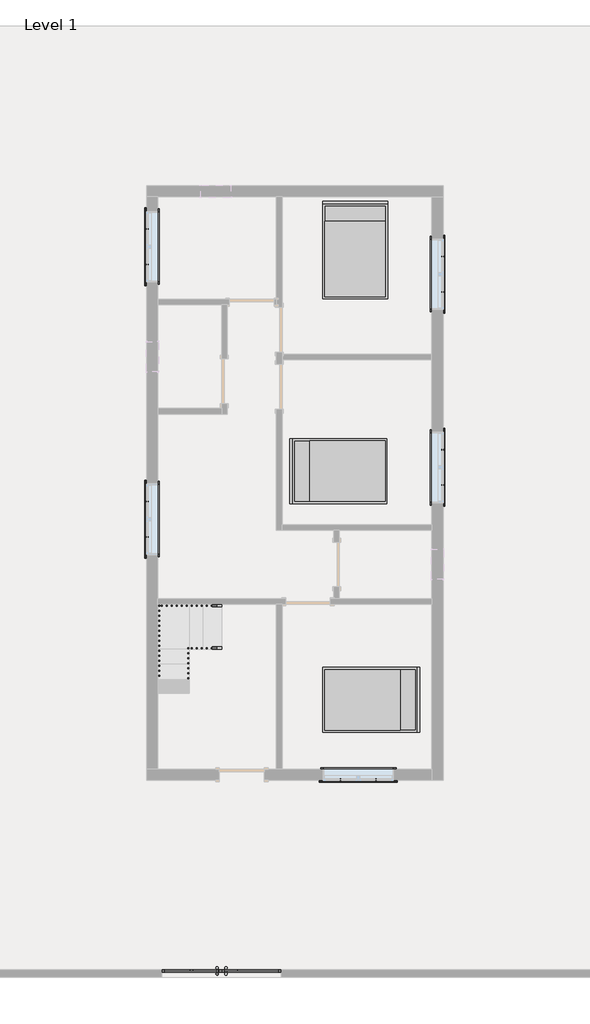
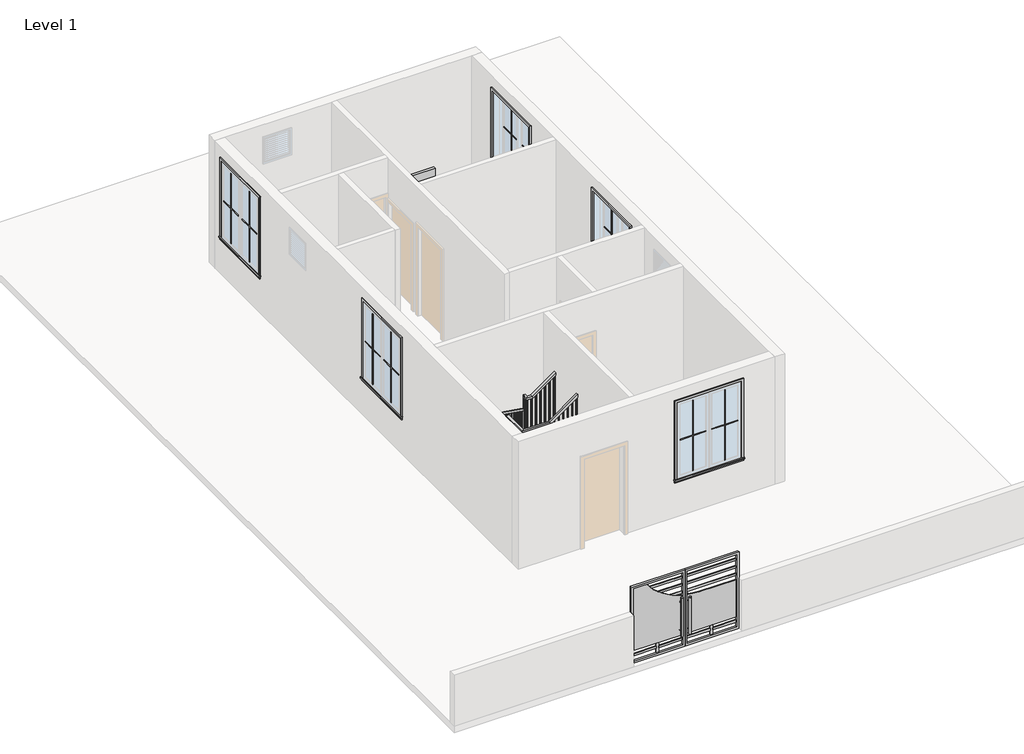
# One storey, part 2 of 2: 21 proxies, 3 furniture elements, 2 railings.
"""IFC4 building model written with IfcOpenShell, lengths in millimetres."""

from ifc_helpers import new_model, si_unit, frame, origin, place, context, project, spatial, polyline, outline, extrude, faceted_brep, transform, mapped, element, save
from components import generic_models_113f6068, muntin_pattern_2x2_muntin_pattern_2x2_bff912c5, muntin_pattern_2x2_muntin_pattern_2x2_c2194282, trim_window_exterior_flat_with_sill_e04b3088, trim_window_interior_flat_picture_frame_2a7685fe, bed_17739_bed_17739_15c61121

model = new_model("IFC4")

# Units and contexts
model_context = context("Model", 3, world=origin())
ifc_project = project(units=[si_unit("LENGTHUNIT", "METRE", prefix="MILLI")], contexts=[model_context])

# Site, building, storey
site = spatial("IfcSite", under=ifc_project)
building = spatial("IfcBuilding", under=site)
storey = spatial("IfcBuildingStorey", under=building, Name="Level 1", Elevation=0.0)

# Proxies
placement = place(None, origin())
generic_models_shape = generic_models_113f6068(model_context)
element("IfcBuildingElementProxy", 1, Name="Generic Models", at=placement, inside=storey, context=model_context, shape_type="MappedRepresentation", body=[
    mapped(generic_models_shape, transform((-2747.4889285, -9775.3328853, 0.0), x_axis=(1.0, 0.0, 0.0), y_axis=(0.0, 1.0, 0.0), z_axis=(0.0, 0.0, 1.0))),
])
muntin_pattern_2x2_muntin_pattern_2x2_shape = muntin_pattern_2x2_muntin_pattern_2x2_bff912c5(model_context)
element("IfcBuildingElementProxy", 2, Name="Muntin Pattern_2x2 : Muntin Pattern_2x2", ObjectType="Muntin Pattern_2x2 : Muntin Pattern_2x2", at=placement, inside=storey, context=model_context, shape_type="MappedRepresentation", body=[
    mapped(muntin_pattern_2x2_muntin_pattern_2x2_shape, transform((-4261.9639285, 4584.2694249, 984.25), x_axis=(0.0, 1.0, 0.0), y_axis=(-1.0, 0.0, 0.0), z_axis=(0.0, 0.0, 1.0))),
])
element("IfcBuildingElementProxy", 3, Name="Muntin Pattern_2x2 : Muntin Pattern_2x2", ObjectType="Muntin Pattern_2x2 : Muntin Pattern_2x2", at=placement, inside=storey, context=model_context, shape_type="MappedRepresentation", body=[
    mapped(muntin_pattern_2x2_muntin_pattern_2x2_shape, transform((1751.4860715, 4746.1944249, 984.25), x_axis=(0.0, -1.0, 0.0), y_axis=(1.0, 0.0, 0.0), z_axis=(0.0, 0.0, 1.0))),
])
element("IfcBuildingElementProxy", 4, Name="Muntin Pattern_2x2 : Muntin Pattern_2x2", ObjectType="Muntin Pattern_2x2 : Muntin Pattern_2x2", at=placement, inside=storey, context=model_context, shape_type="MappedRepresentation", body=[
    mapped(muntin_pattern_2x2_muntin_pattern_2x2_shape, transform((-4261.9639285, -962.4555751, 984.25), x_axis=(0.0, 1.0, 0.0), y_axis=(-1.0, 0.0, 0.0), z_axis=(0.0, 0.0, 1.0))),
])
element("IfcBuildingElementProxy", 5, Name="Muntin Pattern_2x2 : Muntin Pattern_2x2", ObjectType="Muntin Pattern_2x2 : Muntin Pattern_2x2", at=placement, inside=storey, context=model_context, shape_type="MappedRepresentation", body=[
    mapped(muntin_pattern_2x2_muntin_pattern_2x2_shape, transform((1751.4860715, 812.3694249, 984.25), x_axis=(0.0, -1.0, 0.0), y_axis=(1.0, 0.0, 0.0), z_axis=(0.0, 0.0, 1.0))),
])
element("IfcBuildingElementProxy", 6, Name="Muntin Pattern_2x2 : Muntin Pattern_2x2", ObjectType="Muntin Pattern_2x2 : Muntin Pattern_2x2", at=placement, inside=storey, context=model_context, shape_type="MappedRepresentation", body=[
    mapped(muntin_pattern_2x2_muntin_pattern_2x2_shape, transform((397.3485715, -5907.5180751, 984.25), x_axis=(-1.0, 0.0, 0.0), y_axis=(0.0, -1.0, 0.0), z_axis=(0.0, 0.0, 1.0))),
])
muntin_pattern_2x2_muntin_pattern_2x2_2_shape = muntin_pattern_2x2_muntin_pattern_2x2_c2194282(model_context)
element("IfcBuildingElementProxy", 7, Name="Muntin Pattern_2x2 : Muntin Pattern_2x2", ObjectType="Muntin Pattern_2x2 : Muntin Pattern_2x2", at=placement, inside=storey, context=model_context, shape_type="MappedRepresentation", body=[
    mapped(muntin_pattern_2x2_muntin_pattern_2x2_2_shape, transform((-4261.9639285, 5304.9944249, 984.25), x_axis=(0.0, -1.0, 0.0), y_axis=(1.0, 0.0, 0.0), z_axis=(0.0, 0.0, 1.0))),
])
element("IfcBuildingElementProxy", 8, Name="Muntin Pattern_2x2 : Muntin Pattern_2x2", ObjectType="Muntin Pattern_2x2 : Muntin Pattern_2x2", at=placement, inside=storey, context=model_context, shape_type="MappedRepresentation", body=[
    mapped(muntin_pattern_2x2_muntin_pattern_2x2_2_shape, transform((1751.4860715, 4025.4694249, 984.25), x_axis=(0.0, 1.0, 0.0), y_axis=(-1.0, 0.0, 0.0), z_axis=(0.0, 0.0, 1.0))),
])
element("IfcBuildingElementProxy", 9, Name="Muntin Pattern_2x2 : Muntin Pattern_2x2", ObjectType="Muntin Pattern_2x2 : Muntin Pattern_2x2", at=placement, inside=storey, context=model_context, shape_type="MappedRepresentation", body=[
    mapped(muntin_pattern_2x2_muntin_pattern_2x2_2_shape, transform((-4261.9639285, -241.7305751, 984.25), x_axis=(0.0, -1.0, 0.0), y_axis=(1.0, 0.0, 0.0), z_axis=(0.0, 0.0, 1.0))),
])
element("IfcBuildingElementProxy", 10, Name="Muntin Pattern_2x2 : Muntin Pattern_2x2", ObjectType="Muntin Pattern_2x2 : Muntin Pattern_2x2", at=placement, inside=storey, context=model_context, shape_type="MappedRepresentation", body=[
    mapped(muntin_pattern_2x2_muntin_pattern_2x2_2_shape, transform((1751.4860715, 91.6444249, 984.25), x_axis=(0.0, 1.0, 0.0), y_axis=(-1.0, 0.0, 0.0), z_axis=(0.0, 0.0, 1.0))),
])
element("IfcBuildingElementProxy", 11, Name="Muntin Pattern_2x2 : Muntin Pattern_2x2", ObjectType="Muntin Pattern_2x2 : Muntin Pattern_2x2", at=placement, inside=storey, context=model_context, shape_type="MappedRepresentation", body=[
    mapped(muntin_pattern_2x2_muntin_pattern_2x2_2_shape, transform((-323.3764285, -5907.5180751, 984.25), x_axis=(1.0, 0.0, 0.0), y_axis=(0.0, 1.0, 0.0), z_axis=(0.0, 0.0, 1.0))),
])
trim_window_exterior_flat_with_sill_shape = trim_window_exterior_flat_with_sill_e04b3088(model_context)
element("IfcBuildingElementProxy", 12, Name="Trim-Window-Exterior-Flat : with Sill", ObjectType="Trim-Window-Exterior-Flat : with Sill", at=placement, inside=storey, context=model_context, shape_type="MappedRepresentation", body=[
    mapped(trim_window_exterior_flat_with_sill_shape, transform((-4271.4889285, 4944.6319249, 2743.2), x_axis=(0.0, -1.0, 0.0), y_axis=(0.0, 0.0, 1.0), z_axis=(-1.0, 0.0, 0.0))),
])
element("IfcBuildingElementProxy", 13, Name="Trim-Window-Exterior-Flat : with Sill", ObjectType="Trim-Window-Exterior-Flat : with Sill", at=placement, inside=storey, context=model_context, shape_type="MappedRepresentation", body=[
    mapped(trim_window_exterior_flat_with_sill_shape, transform((1761.0110715, 4385.8319249, 2743.2), x_axis=(0.0, 1.0, 0.0), y_axis=(0.0, 0.0, 1.0), z_axis=(1.0, 0.0, 0.0))),
])
element("IfcBuildingElementProxy", 14, Name="Trim-Window-Exterior-Flat : with Sill", ObjectType="Trim-Window-Exterior-Flat : with Sill", at=placement, inside=storey, context=model_context, shape_type="MappedRepresentation", body=[
    mapped(trim_window_exterior_flat_with_sill_shape, transform((-4271.4889285, -602.0930751, 2743.2), x_axis=(0.0, -1.0, 0.0), y_axis=(0.0, 0.0, 1.0), z_axis=(-1.0, 0.0, 0.0))),
])
element("IfcBuildingElementProxy", 15, Name="Trim-Window-Exterior-Flat : with Sill", ObjectType="Trim-Window-Exterior-Flat : with Sill", at=placement, inside=storey, context=model_context, shape_type="MappedRepresentation", body=[
    mapped(trim_window_exterior_flat_with_sill_shape, transform((1761.0110715, 452.0069249, 2743.2), x_axis=(0.0, 1.0, 0.0), y_axis=(0.0, 0.0, 1.0), z_axis=(1.0, 0.0, 0.0))),
])
element("IfcBuildingElementProxy", 16, Name="Trim-Window-Exterior-Flat : with Sill", ObjectType="Trim-Window-Exterior-Flat : with Sill", at=placement, inside=storey, context=model_context, shape_type="MappedRepresentation", body=[
    mapped(trim_window_exterior_flat_with_sill_shape, transform((36.9860715, -5917.0430751, 2743.2), x_axis=(1.0, 0.0, 0.0), y_axis=(0.0, 0.0, 1.0), z_axis=(0.0, -1.0, 0.0))),
])
trim_window_interior_flat_picture_frame_shape = trim_window_interior_flat_picture_frame_2a7685fe(model_context)
element("IfcBuildingElementProxy", 17, Name="Trim-Window-Interior-Flat : Picture Frame", ObjectType="Trim-Window-Interior-Flat : Picture Frame", at=placement, inside=storey, context=model_context, shape_type="MappedRepresentation", body=[
    mapped(trim_window_interior_flat_picture_frame_shape, transform((-4042.8889285, 4944.6319249, 2743.2), x_axis=(0.0, 1.0, 0.0), y_axis=(0.0, 0.0, 1.0), z_axis=(1.0, 0.0, 0.0))),
])
element("IfcBuildingElementProxy", 18, Name="Trim-Window-Interior-Flat : Picture Frame", ObjectType="Trim-Window-Interior-Flat : Picture Frame", at=placement, inside=storey, context=model_context, shape_type="MappedRepresentation", body=[
    mapped(trim_window_interior_flat_picture_frame_shape, transform((1532.4110715, 4385.8319249, 2743.2), x_axis=(0.0, -1.0, 0.0), y_axis=(0.0, 0.0, 1.0), z_axis=(-1.0, 0.0, 0.0))),
])
element("IfcBuildingElementProxy", 19, Name="Trim-Window-Interior-Flat : Picture Frame", ObjectType="Trim-Window-Interior-Flat : Picture Frame", at=placement, inside=storey, context=model_context, shape_type="MappedRepresentation", body=[
    mapped(trim_window_interior_flat_picture_frame_shape, transform((-4042.8889285, -602.0930751, 2743.2), x_axis=(0.0, 1.0, 0.0), y_axis=(0.0, 0.0, 1.0), z_axis=(1.0, 0.0, 0.0))),
])
element("IfcBuildingElementProxy", 20, Name="Trim-Window-Interior-Flat : Picture Frame", ObjectType="Trim-Window-Interior-Flat : Picture Frame", at=placement, inside=storey, context=model_context, shape_type="MappedRepresentation", body=[
    mapped(trim_window_interior_flat_picture_frame_shape, transform((1532.4110715, 452.0069249, 2743.2), x_axis=(0.0, -1.0, 0.0), y_axis=(0.0, 0.0, 1.0), z_axis=(-1.0, 0.0, 0.0))),
])
element("IfcBuildingElementProxy", 21, Name="Trim-Window-Interior-Flat : Picture Frame", ObjectType="Trim-Window-Interior-Flat : Picture Frame", at=placement, inside=storey, context=model_context, shape_type="MappedRepresentation", body=[
    mapped(trim_window_interior_flat_picture_frame_shape, transform((36.9860715, -5688.4430751, 2743.2), x_axis=(-1.0, 0.0, 0.0), y_axis=(0.0, 0.0, 1.0), z_axis=(0.0, 1.0, 0.0))),
])

# Furniture
bed_17739_bed_17739_shape = bed_17739_bed_17739_15c61121(model_context)
element("IfcFurniture", 22, ObjectType="Bed_17739 : Bed_17739", at=placement, inside=storey, context=model_context, shape_type="MappedRepresentation", body=[
    mapped(bed_17739_bed_17739_shape, transform((-29.6889285, 4852.5569249, 0.0), x_axis=(1.0, 0.0, 0.0), y_axis=(0.0, 1.0, 0.0), z_axis=(0.0, 0.0, 1.0))),
])
element("IfcFurniture", 23, ObjectType="Bed_17739 : Bed_17739", at=placement, inside=storey, context=model_context, shape_type="MappedRepresentation", body=[
    mapped(bed_17739_bed_17739_shape, transform((-347.1889285, 375.8069249, 0.0), x_axis=(0.0, 1.0, 0.0), y_axis=(-1.0, 0.0, 0.0), z_axis=(0.0, 0.0, 1.0))),
])
element("IfcFurniture", 24, ObjectType="Bed_17739 : Bed_17739", at=placement, inside=storey, context=model_context, shape_type="MappedRepresentation", body=[
    mapped(bed_17739_bed_17739_shape, transform((275.1110715, -4278.7430751, 0.0), x_axis=(0.0, -1.0, 0.0), y_axis=(1.0, 0.0, 0.0), z_axis=(0.0, 0.0, 1.0))),
])

# Railings
element("IfcRailing", 25, ObjectType="Handrail - Rectangular", at=placement, inside=storey, context=model_context, shape_type="SolidModel", body=[
    faceted_brep([(-2747.4889285, -2386.4430751, 1132.1142857), (-2747.4889285, -2386.4430751, 1071.0863269), (-2747.4889285, -2335.6430751, 1071.0863269), (-2747.4889285, -2335.6430751, 1132.1142857), (-3396.0267484, -2386.4430751, 1563.8731672), (-3411.3899949, -2386.4430751, 1513.0731672), (-3411.3899949, -2335.6430751, 1513.0731672), (-3396.0267484, -2335.6430751, 1563.8731672), (-3992.0889285, -2386.4430751, 1563.8731672), (-3992.0889285, -2386.4430751, 1513.0731672), (-4042.8889285, -2335.6430751, 1513.0731672), (-4042.8889285, -2335.6430751, 1563.8731672), (-3992.0889285, -2940.1628326, 1563.8731672), (-3992.0889285, -2956.4449078, 1513.0731672), (-4042.8889285, -2956.4449078, 1513.0731672), (-4042.8889285, -2940.1628326, 1563.8731672), (-3992.0889285, -5061.9991591, 3079.750907), (-3992.0889285, -5078.2812343, 3028.950907), (-4042.8889285, -5078.2812343, 3028.950907), (-4042.8889285, -5061.9991591, 3079.750907), (-3992.0889285, -5637.6430751, 3079.750907), (-3992.0889285, -5637.6430751, 3028.950907), (-4042.8889285, -5688.4430751, 3028.950907), (-4042.8889285, -5688.4430751, 3079.750907), (-3418.001852, -5637.6430751, 3079.750907), (-3401.6853947, -5637.6430751, 3028.950907), (-3401.6853947, -5688.4430751, 3028.950907), (-3418.001852, -5688.4430751, 3079.750907), (-2793.6303845, -5637.6430751, 3526.9714286), (-2793.6303845, -5688.4430751, 3526.9714286), (-2793.6303845, -5688.4430751, 3464.4843882), (-2793.6303845, -5637.6430751, 3464.4843882)], [[[0, 1, 2, 3]], [[1, 0, 4, 5]], [[2, 1, 5, 6]], [[3, 2, 6, 7]], [[0, 3, 7, 4]], [[5, 4, 8, 9]], [[6, 5, 9, 10]], [[7, 6, 10, 11]], [[4, 7, 11, 8]], [[9, 8, 12, 13]], [[10, 9, 13, 14]], [[11, 10, 14, 15]], [[8, 11, 15, 12]], [[13, 12, 16, 17]], [[14, 13, 17, 18]], [[15, 14, 18, 19]], [[12, 15, 19, 16]], [[17, 16, 20, 21]], [[18, 17, 21, 22]], [[19, 18, 22, 23]], [[16, 19, 23, 20]], [[21, 20, 24, 25]], [[22, 21, 25, 26]], [[23, 22, 26, 27]], [[20, 23, 27, 24]], [[28, 29, 30, 31]], [[25, 24, 28, 31]], [[26, 25, 31, 30]], [[27, 26, 30, 29]], [[24, 27, 29, 28]]]),
    extrude(outline(polyline([(3467.9701, -2788.7639285), (3454.3250964, -2807.8139285), (2394.8571429, -2807.8139285), (2394.8571429, -2788.7639285), (3467.9701, -2788.7639285)])), frame((0.0, -5672.5680751, 0.0), z_axis=(0.0, 1.0, 0.0), x_axis=(0.0, 0.0, 1.0)), (0.0, 0.0, 1.0), 19.05),
    extrude(outline(polyline([(3395.1967474, -2890.3639285), (3381.5517437, -2909.4139285), (2394.8571429, -2909.4139285), (2394.8571429, -2890.3639285), (3395.1967474, -2890.3639285)])), frame((0.0, -5672.5680751, 0.0), z_axis=(0.0, 1.0, 0.0), x_axis=(0.0, 0.0, 1.0)), (0.0, 0.0, 1.0), 19.05),
    extrude(outline(polyline([(3322.4233947, -2991.9639285), (3308.7783911, -3011.0139285), (2394.8571429, -3011.0139285), (2394.8571429, -2991.9639285), (3322.4233947, -2991.9639285)])), frame((0.0, -5672.5680751, 0.0), z_axis=(0.0, 1.0, 0.0), x_axis=(0.0, 0.0, 1.0)), (0.0, 0.0, 1.0), 19.05),
    extrude(outline(polyline([(3249.650042, -3093.5639285), (3236.0050384, -3112.6139285), (2394.8571429, -3112.6139285), (2394.8571429, -3093.5639285), (3249.650042, -3093.5639285)])), frame((0.0, -5672.5680751, 0.0), z_axis=(0.0, 1.0, 0.0), x_axis=(0.0, 0.0, 1.0)), (0.0, 0.0, 1.0), 19.05),
    extrude(outline(polyline([(3176.8766894, -3195.1639285), (3163.2316857, -3214.2139285), (2177.1428571, -3214.2139285), (2177.1428571, -3195.1639285), (3176.8766894, -3195.1639285)])), frame((0.0, -5672.5680751, 0.0), z_axis=(0.0, 1.0, 0.0), x_axis=(0.0, 0.0, 1.0)), (0.0, 0.0, 1.0), 19.05),
    extrude(outline(polyline([(3104.1033367, -3296.7639285), (3090.4583331, -3315.8139285), (2177.1428571, -3315.8139285), (2177.1428571, -3296.7639285), (3104.1033367, -3296.7639285)])), frame((0.0, -5672.5680751, 0.0), z_axis=(0.0, 1.0, 0.0), x_axis=(0.0, 0.0, 1.0)), (0.0, 0.0, 1.0), 19.05),
    extrude(outline(polyline([(3031.329984, -3398.3639285), (3017.6849804, -3417.4139285), (1959.4285714, -3417.4139285), (1959.4285714, -3398.3639285), (3031.329984, -3398.3639285)])), frame((0.0, -5672.5680751, 0.0), z_axis=(0.0, 1.0, 0.0), x_axis=(0.0, 0.0, 1.0)), (0.0, 0.0, 1.0), 19.05),
    extrude(outline(polyline([(-3519.0139285, -5672.5680751), (-3519.0139285, -5653.5180751), (-3499.9639285, -5653.5180751), (-3499.9639285, -5672.5680751), (-3519.0139285, -5672.5680751)])), frame((0.0, 0.0, 1959.4285714), z_axis=(0.0, 0.0, 1.0), x_axis=(1.0, 0.0, 0.0)), (0.0, 0.0, 1.0), 1069.5223355),
    extrude(outline(polyline([(-3620.6139285, -5672.5680751), (-3620.6139285, -5653.5180751), (-3601.5639285, -5653.5180751), (-3601.5639285, -5672.5680751), (-3620.6139285, -5672.5680751)])), frame((0.0, 0.0, 1959.4285714), z_axis=(0.0, 0.0, 1.0), x_axis=(1.0, 0.0, 0.0)), (0.0, 0.0, 1.0), 1069.5223355),
    extrude(outline(polyline([(-3722.2139285, -5672.5680751), (-3722.2139285, -5653.5180751), (-3703.1639285, -5653.5180751), (-3703.1639285, -5672.5680751), (-3722.2139285, -5672.5680751)])), frame((0.0, 0.0, 1959.4285714), z_axis=(0.0, 0.0, 1.0), x_axis=(1.0, 0.0, 0.0)), (0.0, 0.0, 1.0), 1069.5223355),
    extrude(outline(polyline([(-3823.8139285, -5672.5680751), (-3823.8139285, -5653.5180751), (-3804.7639285, -5653.5180751), (-3804.7639285, -5672.5680751), (-3823.8139285, -5672.5680751)])), frame((0.0, 0.0, 1959.4285714), z_axis=(0.0, 0.0, 1.0), x_axis=(1.0, 0.0, 0.0)), (0.0, 0.0, 1.0), 1069.5223355),
    extrude(outline(polyline([(-3925.4139285, -5672.5680751), (-3925.4139285, -5653.5180751), (-3906.3639285, -5653.5180751), (-3906.3639285, -5672.5680751), (-3925.4139285, -5672.5680751)])), frame((0.0, 0.0, 1959.4285714), z_axis=(0.0, 0.0, 1.0), x_axis=(1.0, 0.0, 0.0)), (0.0, 0.0, 1.0), 1069.5223355),
    extrude(outline(polyline([(-4027.0139285, -5602.7180751), (-4007.9639285, -5602.7180751), (-4007.9639285, -5621.7680751), (-4027.0139285, -5621.7680751), (-4027.0139285, -5602.7180751)])), frame((0.0, 0.0, 1959.4285714), z_axis=(0.0, 0.0, 1.0), x_axis=(1.0, 0.0, 0.0)), (0.0, 0.0, 1.0), 1069.5223355),
    extrude(outline(polyline([(-4027.0139285, -5501.1180751), (-4007.9639285, -5501.1180751), (-4007.9639285, -5520.1680751), (-4027.0139285, -5520.1680751), (-4027.0139285, -5501.1180751)])), frame((0.0, 0.0, 1959.4285714), z_axis=(0.0, 0.0, 1.0), x_axis=(1.0, 0.0, 0.0)), (0.0, 0.0, 1.0), 1069.5223355),
    extrude(outline(polyline([(-4027.0139285, -5399.5180751), (-4007.9639285, -5399.5180751), (-4007.9639285, -5418.5680751), (-4027.0139285, -5418.5680751), (-4027.0139285, -5399.5180751)])), frame((0.0, 0.0, 1959.4285714), z_axis=(0.0, 0.0, 1.0), x_axis=(1.0, 0.0, 0.0)), (0.0, 0.0, 1.0), 1069.5223355),
    extrude(outline(polyline([(-4027.0139285, -5297.9180751), (-4007.9639285, -5297.9180751), (-4007.9639285, -5316.9680751), (-4027.0139285, -5316.9680751), (-4027.0139285, -5297.9180751)])), frame((0.0, 0.0, 1959.4285714), z_axis=(0.0, 0.0, 1.0), x_axis=(1.0, 0.0, 0.0)), (0.0, 0.0, 1.0), 1069.5223355),
    extrude(outline(polyline([(-4027.0139285, -5196.3180751), (-4007.9639285, -5196.3180751), (-4007.9639285, -5215.3680751), (-4027.0139285, -5215.3680751), (-4027.0139285, -5196.3180751)])), frame((0.0, 0.0, 1959.4285714), z_axis=(0.0, 0.0, 1.0), x_axis=(1.0, 0.0, 0.0)), (0.0, 0.0, 1.0), 1069.5223355),
    extrude(outline(polyline([(-4027.0139285, -5094.7180751), (-4007.9639285, -5094.7180751), (-4007.9639285, -5113.7680751), (-4027.0139285, -5113.7680751), (-4027.0139285, -5094.7180751)])), frame((0.0, 0.0, 1959.4285714), z_axis=(0.0, 0.0, 1.0), x_axis=(1.0, 0.0, 0.0)), (0.0, 0.0, 1.0), 1069.5223355),
    extrude(outline(polyline([(-5012.1680751, 2981.6379382), (-4993.1180751, 2968.0282782), (-4993.1180751, 1959.4285714), (-5012.1680751, 1959.4285714), (-5012.1680751, 2981.6379382)])), frame((-4027.0139285, 0.0, 0.0), z_axis=(1.0, 0.0, 0.0), x_axis=(0.0, 1.0, 0.0)), (0.0, 0.0, 1.0), 19.05),
    extrude(outline(polyline([(-4910.5680751, 2909.0530849), (-4891.5180751, 2895.4434249), (-4891.5180751, 1959.4285714), (-4910.5680751, 1959.4285714), (-4910.5680751, 2909.0530849)])), frame((-4027.0139285, 0.0, 0.0), z_axis=(1.0, 0.0, 0.0), x_axis=(0.0, 1.0, 0.0)), (0.0, 0.0, 1.0), 19.05),
    extrude(outline(polyline([(-4808.9680751, 2836.4682317), (-4789.9180751, 2822.8585717), (-4789.9180751, 1959.4285714), (-4808.9680751, 1959.4285714), (-4808.9680751, 2836.4682317)])), frame((-4027.0139285, 0.0, 0.0), z_axis=(1.0, 0.0, 0.0), x_axis=(0.0, 1.0, 0.0)), (0.0, 0.0, 1.0), 19.05),
    extrude(outline(polyline([(-4707.3680751, 2763.9236524), (-4688.3180751, 2750.3139925), (-4688.3180751, 1741.7142857), (-4707.3680751, 1741.7142857), (-4707.3680751, 2763.9236524)])), frame((-4027.0139285, 0.0, 0.0), z_axis=(1.0, 0.0, 0.0), x_axis=(0.0, 1.0, 0.0)), (0.0, 0.0, 1.0), 19.05),
    extrude(outline(polyline([(-4605.7680751, 2691.3387992), (-4586.7180751, 2677.7291392), (-4586.7180751, 1741.7142857), (-4605.7680751, 1741.7142857), (-4605.7680751, 2691.3387992)])), frame((-4027.0139285, 0.0, 0.0), z_axis=(1.0, 0.0, 0.0), x_axis=(0.0, 1.0, 0.0)), (0.0, 0.0, 1.0), 19.05),
    extrude(outline(polyline([(-4504.1680751, 2618.753946), (-4485.1180751, 2605.144286), (-4485.1180751, 1741.7142857), (-4504.1680751, 1741.7142857), (-4504.1680751, 2618.753946)])), frame((-4027.0139285, 0.0, 0.0), z_axis=(1.0, 0.0, 0.0), x_axis=(0.0, 1.0, 0.0)), (0.0, 0.0, 1.0), 19.05),
    extrude(outline(polyline([(-4402.5680751, 2546.2093667), (-4383.5180751, 2532.5997067), (-4383.5180751, 1524.0), (-4402.5680751, 1524.0), (-4402.5680751, 2546.2093667)])), frame((-4027.0139285, 0.0, 0.0), z_axis=(1.0, 0.0, 0.0), x_axis=(0.0, 1.0, 0.0)), (0.0, 0.0, 1.0), 19.05),
    extrude(outline(polyline([(-4300.9680751, 2473.6245135), (-4281.9180751, 2460.0148535), (-4281.9180751, 1524.0), (-4300.9680751, 1524.0), (-4300.9680751, 2473.6245135)])), frame((-4027.0139285, 0.0, 0.0), z_axis=(1.0, 0.0, 0.0), x_axis=(0.0, 1.0, 0.0)), (0.0, 0.0, 1.0), 19.05),
    extrude(outline(polyline([(-4199.3680751, 2401.0396602), (-4180.3180751, 2387.4300003), (-4180.3180751, 1524.0), (-4199.3680751, 1524.0), (-4199.3680751, 2401.0396602)])), frame((-4027.0139285, 0.0, 0.0), z_axis=(1.0, 0.0, 0.0), x_axis=(0.0, 1.0, 0.0)), (0.0, 0.0, 1.0), 19.05),
    extrude(outline(polyline([(-4097.7680751, 2328.333985), (-4078.7180751, 2314.724325), (-4078.7180751, 1306.2857143), (-4097.7680751, 1306.2857143), (-4097.7680751, 2328.333985)])), frame((-4027.0139285, 0.0, 0.0), z_axis=(1.0, 0.0, 0.0), x_axis=(0.0, 1.0, 0.0)), (0.0, 0.0, 1.0), 19.05),
    extrude(outline(polyline([(-3996.1680751, 2255.7491318), (-3977.1180751, 2242.1394718), (-3977.1180751, 1306.2857143), (-3996.1680751, 1306.2857143), (-3996.1680751, 2255.7491318)])), frame((-4027.0139285, 0.0, 0.0), z_axis=(1.0, 0.0, 0.0), x_axis=(0.0, 1.0, 0.0)), (0.0, 0.0, 1.0), 19.05),
    extrude(outline(polyline([(-3894.5680751, 2183.1642785), (-3875.5180751, 2169.5546185), (-3875.5180751, 1306.2857143), (-3894.5680751, 1306.2857143), (-3894.5680751, 2183.1642785)])), frame((-4027.0139285, 0.0, 0.0), z_axis=(1.0, 0.0, 0.0), x_axis=(0.0, 1.0, 0.0)), (0.0, 0.0, 1.0), 19.05),
    extrude(outline(polyline([(-3792.9680751, 2110.6196993), (-3773.9180751, 2097.0100393), (-3773.9180751, 1088.5714286), (-3792.9680751, 1088.5714286), (-3792.9680751, 2110.6196993)])), frame((-4027.0139285, 0.0, 0.0), z_axis=(1.0, 0.0, 0.0), x_axis=(0.0, 1.0, 0.0)), (0.0, 0.0, 1.0), 19.05),
    extrude(outline(polyline([(-3691.3680751, 2038.034846), (-3672.3180751, 2024.4251861), (-3672.3180751, 1088.5714286), (-3691.3680751, 1088.5714286), (-3691.3680751, 2038.034846)])), frame((-4027.0139285, 0.0, 0.0), z_axis=(1.0, 0.0, 0.0), x_axis=(0.0, 1.0, 0.0)), (0.0, 0.0, 1.0), 19.05),
    extrude(outline(polyline([(-3589.7680751, 1965.4499928), (-3570.7180751, 1951.8403328), (-3570.7180751, 1088.5714286), (-3589.7680751, 1088.5714286), (-3589.7680751, 1965.4499928)])), frame((-4027.0139285, 0.0, 0.0), z_axis=(1.0, 0.0, 0.0), x_axis=(0.0, 1.0, 0.0)), (0.0, 0.0, 1.0), 19.05),
    extrude(outline(polyline([(-3488.1680751, 1892.9054136), (-3469.1180751, 1879.2957536), (-3469.1180751, 870.8571429), (-3488.1680751, 870.8571429), (-3488.1680751, 1892.9054136)])), frame((-4027.0139285, 0.0, 0.0), z_axis=(1.0, 0.0, 0.0), x_axis=(0.0, 1.0, 0.0)), (0.0, 0.0, 1.0), 19.05),
    extrude(outline(polyline([(-3386.5680751, 1820.3205603), (-3367.5180751, 1806.7109003), (-3367.5180751, 870.8571429), (-3386.5680751, 870.8571429), (-3386.5680751, 1820.3205603)])), frame((-4027.0139285, 0.0, 0.0), z_axis=(1.0, 0.0, 0.0), x_axis=(0.0, 1.0, 0.0)), (0.0, 0.0, 1.0), 19.05),
    extrude(outline(polyline([(-3284.9680751, 1747.7357071), (-3265.9180751, 1734.1260471), (-3265.9180751, 870.8571429), (-3284.9680751, 870.8571429), (-3284.9680751, 1747.7357071)])), frame((-4027.0139285, 0.0, 0.0), z_axis=(1.0, 0.0, 0.0), x_axis=(0.0, 1.0, 0.0)), (0.0, 0.0, 1.0), 19.05),
    extrude(outline(polyline([(-3183.3680751, 1675.1911278), (-3164.3180751, 1661.5814679), (-3164.3180751, 653.1428571), (-3183.3680751, 653.1428571), (-3183.3680751, 1675.1911278)])), frame((-4027.0139285, 0.0, 0.0), z_axis=(1.0, 0.0, 0.0), x_axis=(0.0, 1.0, 0.0)), (0.0, 0.0, 1.0), 19.05),
    extrude(outline(polyline([(-3081.7680751, 1602.6062746), (-3062.7180751, 1588.9966146), (-3062.7180751, 653.1428571), (-3081.7680751, 653.1428571), (-3081.7680751, 1602.6062746)])), frame((-4027.0139285, 0.0, 0.0), z_axis=(1.0, 0.0, 0.0), x_axis=(0.0, 1.0, 0.0)), (0.0, 0.0, 1.0), 19.05),
    extrude(outline(polyline([(-2980.1680751, 1530.0214214), (-2961.1180751, 1516.4117614), (-2961.1180751, 653.1428571), (-2980.1680751, 653.1428571), (-2980.1680751, 1530.0214214)])), frame((-4027.0139285, 0.0, 0.0), z_axis=(1.0, 0.0, 0.0), x_axis=(0.0, 1.0, 0.0)), (0.0, 0.0, 1.0), 19.05),
    extrude(outline(polyline([(-4027.0139285, -2859.5180751), (-4007.9639285, -2859.5180751), (-4007.9639285, -2878.5680751), (-4027.0139285, -2878.5680751), (-4027.0139285, -2859.5180751)])), frame((0.0, 0.0, 653.1428571), z_axis=(0.0, 0.0, 1.0), x_axis=(1.0, 0.0, 0.0)), (0.0, 0.0, 1.0), 859.9303101),
    extrude(outline(polyline([(-4027.0139285, -2757.9180751), (-4007.9639285, -2757.9180751), (-4007.9639285, -2776.9680751), (-4027.0139285, -2776.9680751), (-4027.0139285, -2757.9180751)])), frame((0.0, 0.0, 653.1428571), z_axis=(0.0, 0.0, 1.0), x_axis=(1.0, 0.0, 0.0)), (0.0, 0.0, 1.0), 859.9303101),
    extrude(outline(polyline([(-4027.0139285, -2656.3180751), (-4007.9639285, -2656.3180751), (-4007.9639285, -2675.3680751), (-4027.0139285, -2675.3680751), (-4027.0139285, -2656.3180751)])), frame((0.0, 0.0, 653.1428571), z_axis=(0.0, 0.0, 1.0), x_axis=(1.0, 0.0, 0.0)), (0.0, 0.0, 1.0), 859.9303101),
    extrude(outline(polyline([(-4027.0139285, -2554.7180751), (-4007.9639285, -2554.7180751), (-4007.9639285, -2573.7680751), (-4027.0139285, -2573.7680751), (-4027.0139285, -2554.7180751)])), frame((0.0, 0.0, 653.1428571), z_axis=(0.0, 0.0, 1.0), x_axis=(1.0, 0.0, 0.0)), (0.0, 0.0, 1.0), 859.9303101),
    extrude(outline(polyline([(-4027.0139285, -2453.1180751), (-4007.9639285, -2453.1180751), (-4007.9639285, -2472.1680751), (-4027.0139285, -2472.1680751), (-4027.0139285, -2453.1180751)])), frame((0.0, 0.0, 653.1428571), z_axis=(0.0, 0.0, 1.0), x_axis=(1.0, 0.0, 0.0)), (0.0, 0.0, 1.0), 859.9303101),
    extrude(outline(polyline([(-3957.1639285, -2351.5180751), (-3957.1639285, -2370.5680751), (-3976.2139285, -2370.5680751), (-3976.2139285, -2351.5180751), (-3957.1639285, -2351.5180751)])), frame((0.0, 0.0, 653.1428571), z_axis=(0.0, 0.0, 1.0), x_axis=(1.0, 0.0, 0.0)), (0.0, 0.0, 1.0), 859.9303101),
    extrude(outline(polyline([(-3855.5639285, -2351.5180751), (-3855.5639285, -2370.5680751), (-3874.6139285, -2370.5680751), (-3874.6139285, -2351.5180751), (-3855.5639285, -2351.5180751)])), frame((0.0, 0.0, 653.1428571), z_axis=(0.0, 0.0, 1.0), x_axis=(1.0, 0.0, 0.0)), (0.0, 0.0, 1.0), 859.9303101),
    extrude(outline(polyline([(-3753.9639285, -2351.5180751), (-3753.9639285, -2370.5680751), (-3773.0139285, -2370.5680751), (-3773.0139285, -2351.5180751), (-3753.9639285, -2351.5180751)])), frame((0.0, 0.0, 653.1428571), z_axis=(0.0, 0.0, 1.0), x_axis=(1.0, 0.0, 0.0)), (0.0, 0.0, 1.0), 859.9303101),
    extrude(outline(polyline([(-3652.3639285, -2351.5180751), (-3652.3639285, -2370.5680751), (-3671.4139285, -2370.5680751), (-3671.4139285, -2351.5180751), (-3652.3639285, -2351.5180751)])), frame((0.0, 0.0, 653.1428571), z_axis=(0.0, 0.0, 1.0), x_axis=(1.0, 0.0, 0.0)), (0.0, 0.0, 1.0), 859.9303101),
    extrude(outline(polyline([(-3550.7639285, -2351.5180751), (-3550.7639285, -2370.5680751), (-3569.8139285, -2370.5680751), (-3569.8139285, -2351.5180751), (-3550.7639285, -2351.5180751)])), frame((0.0, 0.0, 653.1428571), z_axis=(0.0, 0.0, 1.0), x_axis=(1.0, 0.0, 0.0)), (0.0, 0.0, 1.0), 859.9303101),
    extrude(outline(polyline([(-3449.1639285, -2351.5180751), (-3449.1639285, -2370.5680751), (-3468.2139285, -2370.5680751), (-3468.2139285, -2351.5180751), (-3449.1639285, -2351.5180751)])), frame((0.0, 0.0, 653.1428571), z_axis=(0.0, 0.0, 1.0), x_axis=(1.0, 0.0, 0.0)), (0.0, 0.0, 1.0), 859.9303101),
    extrude(outline(polyline([(1470.5814725, -3347.5639285), (1483.2638581, -3366.6139285), (435.4285714, -3366.6139285), (435.4285714, -3347.5639285), (1470.5814725, -3347.5639285)])), frame((0.0, -2370.5680751, 0.0), z_axis=(0.0, 1.0, 0.0), x_axis=(0.0, 0.0, 1.0)), (0.0, 0.0, 1.0), 19.05),
    extrude(outline(polyline([(1402.9420828, -3245.9639285), (1415.6244683, -3265.0139285), (435.4285714, -3265.0139285), (435.4285714, -3245.9639285), (1402.9420828, -3245.9639285)])), frame((0.0, -2370.5680751, 0.0), z_axis=(0.0, 1.0, 0.0), x_axis=(0.0, 0.0, 1.0)), (0.0, 0.0, 1.0), 19.05),
    extrude(outline(polyline([(1335.302693, -3144.3639285), (1347.9850786, -3163.4139285), (435.4285714, -3163.4139285), (435.4285714, -3144.3639285), (1335.302693, -3144.3639285)])), frame((0.0, -2370.5680751, 0.0), z_axis=(0.0, 1.0, 0.0), x_axis=(0.0, 0.0, 1.0)), (0.0, 0.0, 1.0), 19.05),
    extrude(outline(polyline([(1267.6633033, -3042.7639285), (1280.3456889, -3061.8139285), (217.7142857, -3061.8139285), (217.7142857, -3042.7639285), (1267.6633033, -3042.7639285)])), frame((0.0, -2370.5680751, 0.0), z_axis=(0.0, 1.0, 0.0), x_axis=(0.0, 0.0, 1.0)), (0.0, 0.0, 1.0), 19.05),
    extrude(outline(polyline([(1200.0239136, -2941.1639285), (1212.7062991, -2960.2139285), (217.7142857, -2960.2139285), (217.7142857, -2941.1639285), (1200.0239136, -2941.1639285)])), frame((0.0, -2370.5680751, 0.0), z_axis=(0.0, 1.0, 0.0), x_axis=(0.0, 0.0, 1.0)), (0.0, 0.0, 1.0), 19.05),
    extrude(outline(polyline([(1132.3845238, -2839.5639285), (1145.0669094, -2858.6139285), (217.7142857, -2858.6139285), (217.7142857, -2839.5639285), (1132.3845238, -2839.5639285)])), frame((0.0, -2370.5680751, 0.0), z_axis=(0.0, 1.0, 0.0), x_axis=(0.0, 0.0, 1.0)), (0.0, 0.0, 1.0), 19.05),
    extrude(outline(polyline([(-4027.0139285, -5653.5180751), (-4007.9639285, -5653.5180751), (-4007.9639285, -5672.5680751), (-4027.0139285, -5672.5680751), (-4027.0139285, -5653.5180751)])), frame((0.0, 0.0, 1959.4285714), z_axis=(0.0, 0.0, 1.0), x_axis=(1.0, 0.0, 0.0)), (0.0, 0.0, 1.0), 1069.5223355),
    extrude(outline(polyline([(-4007.9639285, -2351.5180751), (-4007.9639285, -2370.5680751), (-4027.0139285, -2370.5680751), (-4027.0139285, -2351.5180751), (-4007.9639285, -2351.5180751)])), frame((0.0, 0.0, 653.1428571), z_axis=(0.0, 0.0, 1.0), x_axis=(1.0, 0.0, 0.0)), (0.0, 0.0, 1.0), 859.9303101),
    extrude(outline(polyline([(3464.4843882, -2793.6303845), (3450.8393846, -2812.6803845), (2394.8571429, -2812.6803845), (2394.8571429, -2793.6303845), (3464.4843882, -2793.6303845)])), frame((0.0, -5672.5680751, 0.0), z_axis=(0.0, 1.0, 0.0), x_axis=(0.0, 0.0, 1.0)), (0.0, 0.0, 1.0), 19.05),
    extrude(outline(polyline([(1071.0863269, -2747.4889285), (1083.7687124, -2766.5389285), (217.7142857, -2766.5389285), (217.7142857, -2747.4889285), (1071.0863269, -2747.4889285)])), frame((0.0, -2370.5680751, 0.0), z_axis=(0.0, 1.0, 0.0), x_axis=(0.0, 0.0, 1.0)), (0.0, 0.0, 1.0), 19.05),
])
element("IfcRailing", 26, ObjectType="Handrail - Rectangular", at=placement, inside=storey, context=model_context, shape_type="SolidModel", body=[
    faceted_brep([(-2747.4889285, -3250.0430751, 1132.1142857), (-2747.4889285, -3250.0430751, 1071.0863269), (-2747.4889285, -3199.2430751, 1071.0863269), (-2747.4889285, -3199.2430751, 1132.1142857), (-3325.3389285, -3250.0430751, 1516.8133148), (-3376.1389285, -3250.0430751, 1489.6050509), (-3376.1389285, -3199.2430751, 1489.6050509), (-3325.3389285, -3199.2430751, 1516.8133148), (-3325.3389285, -3250.0430751, 1839.6957828), (-3376.1389285, -3250.0430751, 1788.8957828), (-3376.1389285, -3199.2430751, 1788.8957828), (-3325.3389285, -3199.2430751, 1839.6957828), (-3401.5389285, -3250.0430751, 1839.6957828), (-3401.5389285, -3250.0430751, 1788.8957828), (-3452.3389285, -3199.2430751, 1788.8957828), (-3452.3389285, -3199.2430751, 1839.6957828), (-3401.5389285, -3326.2430751, 1839.6957828), (-3401.5389285, -3342.5251503, 1788.8957828), (-3452.3389285, -3342.5251503, 1788.8957828), (-3452.3389285, -3326.2430751, 1839.6957828), (-3401.5389285, -4697.5612092, 2819.3899315), (-3401.5389285, -4748.3612092, 2793.250153), (-3452.3389285, -4748.3612092, 2793.250153), (-3452.3389285, -4697.5612092, 2819.3899315), (-3401.5389285, -4697.5612092, 3146.1228716), (-3401.5389285, -4748.3612092, 3095.3228716), (-3452.3389285, -4748.3612092, 3095.3228716), (-3452.3389285, -4697.5612092, 3146.1228716), (-3401.5389285, -4773.7612092, 3146.1228716), (-3401.5389285, -4773.7612092, 3095.3228716), (-3452.3389285, -4824.5612092, 3095.3228716), (-3452.3389285, -4824.5612092, 3146.1228716), (-3325.3389285, -4773.7612092, 3146.1228716), (-3309.0224712, -4773.7612092, 3095.3228716), (-3309.0224712, -4824.5612092, 3095.3228716), (-3325.3389285, -4824.5612092, 3146.1228716), (-2793.6303845, -4773.7612092, 3526.9714286), (-2793.6303845, -4824.5612092, 3526.9714286), (-2793.6303845, -4824.5612092, 3464.4843882), (-2793.6303845, -4773.7612092, 3464.4843882)], [[[0, 1, 2, 3]], [[1, 0, 4, 5]], [[2, 1, 5, 6]], [[3, 2, 6, 7]], [[0, 3, 7, 4]], [[5, 4, 8, 9]], [[6, 5, 9, 10]], [[7, 6, 10, 11]], [[4, 7, 11, 8]], [[9, 8, 12, 13]], [[10, 9, 13, 14]], [[11, 10, 14, 15]], [[8, 11, 15, 12]], [[13, 12, 16, 17]], [[14, 13, 17, 18]], [[15, 14, 18, 19]], [[12, 15, 19, 16]], [[17, 16, 20, 21]], [[18, 17, 21, 22]], [[19, 18, 22, 23]], [[16, 19, 23, 20]], [[21, 20, 24, 25]], [[22, 21, 25, 26]], [[23, 22, 26, 27]], [[20, 23, 27, 24]], [[25, 24, 28, 29]], [[26, 25, 29, 30]], [[27, 26, 30, 31]], [[24, 27, 31, 28]], [[29, 28, 32, 33]], [[30, 29, 33, 34]], [[31, 30, 34, 35]], [[28, 31, 35, 32]], [[36, 37, 38, 39]], [[33, 32, 36, 39]], [[34, 33, 39, 38]], [[35, 34, 38, 37]], [[32, 35, 37, 36]]]),
    extrude(outline(polyline([(3440.6800928, -2826.8639285), (2394.8571429, -2826.8639285), (2394.8571429, -2807.8139285), (3454.3250964, -2807.8139285), (3440.6800928, -2826.8639285)])), frame((0.0, -4808.6862092, 0.0), z_axis=(0.0, 1.0, 0.0), x_axis=(0.0, 0.0, 1.0)), (0.0, 0.0, 1.0), 19.05),
    extrude(outline(polyline([(3367.9067401, -2928.4639285), (2394.8571429, -2928.4639285), (2394.8571429, -2909.4139285), (3381.5517437, -2909.4139285), (3367.9067401, -2928.4639285)])), frame((0.0, -4808.6862092, 0.0), z_axis=(0.0, 1.0, 0.0), x_axis=(0.0, 0.0, 1.0)), (0.0, 0.0, 1.0), 19.05),
    extrude(outline(polyline([(3295.1333874, -3030.0639285), (2394.8571429, -3030.0639285), (2394.8571429, -3011.0139285), (3308.7783911, -3011.0139285), (3295.1333874, -3030.0639285)])), frame((0.0, -4808.6862092, 0.0), z_axis=(0.0, 1.0, 0.0), x_axis=(0.0, 0.0, 1.0)), (0.0, 0.0, 1.0), 19.05),
    extrude(outline(polyline([(3222.3600348, -3131.6639285), (2394.8571429, -3131.6639285), (2394.8571429, -3112.6139285), (3236.0050384, -3112.6139285), (3222.3600348, -3131.6639285)])), frame((0.0, -4808.6862092, 0.0), z_axis=(0.0, 1.0, 0.0), x_axis=(0.0, 0.0, 1.0)), (0.0, 0.0, 1.0), 19.05),
    extrude(outline(polyline([(3149.4904113, -3233.2639285), (2177.1428571, -3233.2639285), (2177.1428571, -3214.2139285), (3163.1000713, -3214.2139285), (3149.4904113, -3233.2639285)])), frame((0.0, -4808.6862092, 0.0), z_axis=(0.0, 1.0, 0.0), x_axis=(0.0, 0.0, 1.0)), (0.0, 0.0, 1.0), 19.05),
    extrude(outline(polyline([(3076.905558, -3334.8639285), (2177.1428571, -3334.8639285), (2177.1428571, -3315.8139285), (3090.515218, -3315.8139285), (3076.905558, -3334.8639285)])), frame((0.0, -4808.6862092, 0.0), z_axis=(0.0, 1.0, 0.0), x_axis=(0.0, 0.0, 1.0)), (0.0, 0.0, 1.0), 19.05),
    extrude(outline(polyline([(-3417.4139285, -4739.1180751), (-3417.4139285, -4758.1680751), (-3436.4639285, -4758.1680751), (-3436.4639285, -4739.1180751), (-3417.4139285, -4739.1180751)])), frame((0.0, 0.0, 1741.7142857), z_axis=(0.0, 0.0, 1.0), x_axis=(1.0, 0.0, 0.0)), (0.0, 0.0, 1.0), 1353.6085859),
    extrude(outline(polyline([(-4637.5180751, 2714.0618398), (-4637.5180751, 1741.7142857), (-4656.5680751, 1741.7142857), (-4656.5680751, 2727.6714998), (-4637.5180751, 2714.0618398)])), frame((-3436.4639285, 0.0, 0.0), z_axis=(1.0, 0.0, 0.0), x_axis=(0.0, 1.0, 0.0)), (0.0, 0.0, 1.0), 19.05),
    extrude(outline(polyline([(-4535.9180751, 2641.4769866), (-4535.9180751, 1741.7142857), (-4554.9680751, 1741.7142857), (-4554.9680751, 2655.0866466), (-4535.9180751, 2641.4769866)])), frame((-3436.4639285, 0.0, 0.0), z_axis=(1.0, 0.0, 0.0), x_axis=(0.0, 1.0, 0.0)), (0.0, 0.0, 1.0), 19.05),
    extrude(outline(polyline([(-4434.3180751, 2568.7713113), (-4434.3180751, 1524.0), (-4453.3680751, 1524.0), (-4453.3680751, 2582.3809713), (-4434.3180751, 2568.7713113)])), frame((-3436.4639285, 0.0, 0.0), z_axis=(1.0, 0.0, 0.0), x_axis=(0.0, 1.0, 0.0)), (0.0, 0.0, 1.0), 19.05),
    extrude(outline(polyline([(-4332.7180751, 2496.1864581), (-4332.7180751, 1524.0), (-4351.7680751, 1524.0), (-4351.7680751, 2509.7961181), (-4332.7180751, 2496.1864581)])), frame((-3436.4639285, 0.0, 0.0), z_axis=(1.0, 0.0, 0.0), x_axis=(0.0, 1.0, 0.0)), (0.0, 0.0, 1.0), 19.05),
    extrude(outline(polyline([(-4231.1180751, 2423.6016049), (-4231.1180751, 1524.0), (-4250.1680751, 1524.0), (-4250.1680751, 2437.2112649), (-4231.1180751, 2423.6016049)])), frame((-3436.4639285, 0.0, 0.0), z_axis=(1.0, 0.0, 0.0), x_axis=(0.0, 1.0, 0.0)), (0.0, 0.0, 1.0), 19.05),
    extrude(outline(polyline([(-4129.5180751, 2351.0570256), (-4129.5180751, 1306.2857143), (-4148.5680751, 1306.2857143), (-4148.5680751, 2364.6666856), (-4129.5180751, 2351.0570256)])), frame((-3436.4639285, 0.0, 0.0), z_axis=(1.0, 0.0, 0.0), x_axis=(0.0, 1.0, 0.0)), (0.0, 0.0, 1.0), 19.05),
    extrude(outline(polyline([(-4027.9180751, 2278.4721724), (-4027.9180751, 1306.2857143), (-4046.9680751, 1306.2857143), (-4046.9680751, 2292.0818324), (-4027.9180751, 2278.4721724)])), frame((-3436.4639285, 0.0, 0.0), z_axis=(1.0, 0.0, 0.0), x_axis=(0.0, 1.0, 0.0)), (0.0, 0.0, 1.0), 19.05),
    extrude(outline(polyline([(-3926.3180751, 2205.8873192), (-3926.3180751, 1306.2857143), (-3945.3680751, 1306.2857143), (-3945.3680751, 2219.4969791), (-3926.3180751, 2205.8873192)])), frame((-3436.4639285, 0.0, 0.0), z_axis=(1.0, 0.0, 0.0), x_axis=(0.0, 1.0, 0.0)), (0.0, 0.0, 1.0), 19.05),
    extrude(outline(polyline([(-3824.7180751, 2133.3427399), (-3824.7180751, 1088.5714286), (-3843.7680751, 1088.5714286), (-3843.7680751, 2146.9523999), (-3824.7180751, 2133.3427399)])), frame((-3436.4639285, 0.0, 0.0), z_axis=(1.0, 0.0, 0.0), x_axis=(0.0, 1.0, 0.0)), (0.0, 0.0, 1.0), 19.05),
    extrude(outline(polyline([(-3723.1180751, 2060.7578867), (-3723.1180751, 1088.5714286), (-3742.1680751, 1088.5714286), (-3742.1680751, 2074.3675467), (-3723.1180751, 2060.7578867)])), frame((-3436.4639285, 0.0, 0.0), z_axis=(1.0, 0.0, 0.0), x_axis=(0.0, 1.0, 0.0)), (0.0, 0.0, 1.0), 19.05),
    extrude(outline(polyline([(-3621.5180751, 1988.1730334), (-3621.5180751, 1088.5714286), (-3640.5680751, 1088.5714286), (-3640.5680751, 2001.7826934), (-3621.5180751, 1988.1730334)])), frame((-3436.4639285, 0.0, 0.0), z_axis=(1.0, 0.0, 0.0), x_axis=(0.0, 1.0, 0.0)), (0.0, 0.0, 1.0), 19.05),
    extrude(outline(polyline([(-3519.9180751, 1915.6284542), (-3519.9180751, 870.8571429), (-3538.9680751, 870.8571429), (-3538.9680751, 1929.2381142), (-3519.9180751, 1915.6284542)])), frame((-3436.4639285, 0.0, 0.0), z_axis=(1.0, 0.0, 0.0), x_axis=(0.0, 1.0, 0.0)), (0.0, 0.0, 1.0), 19.05),
    extrude(outline(polyline([(-3418.3180751, 1843.043601), (-3418.3180751, 870.8571429), (-3437.3680751, 870.8571429), (-3437.3680751, 1856.6532609), (-3418.3180751, 1843.043601)])), frame((-3436.4639285, 0.0, 0.0), z_axis=(1.0, 0.0, 0.0), x_axis=(0.0, 1.0, 0.0)), (0.0, 0.0, 1.0), 19.05),
    extrude(outline(polyline([(-3316.7180751, 1770.4587477), (-3316.7180751, 870.8571429), (-3335.7680751, 870.8571429), (-3335.7680751, 1784.0684077), (-3316.7180751, 1770.4587477)])), frame((-3436.4639285, 0.0, 0.0), z_axis=(1.0, 0.0, 0.0), x_axis=(0.0, 1.0, 0.0)), (0.0, 0.0, 1.0), 19.05),
    extrude(outline(polyline([(-3347.5639285, -3234.1680751), (-3366.6139285, -3234.1680751), (-3366.6139285, -3215.1180751), (-3347.5639285, -3215.1180751), (-3347.5639285, -3234.1680751)])), frame((0.0, 0.0, 435.4285714), z_axis=(0.0, 0.0, 1.0), x_axis=(1.0, 0.0, 0.0)), (0.0, 0.0, 1.0), 1353.4672114),
    extrude(outline(polyline([(1415.6244683, -3265.0139285), (435.4285714, -3265.0139285), (435.4285714, -3245.9639285), (1402.9420828, -3245.9639285), (1415.6244683, -3265.0139285)])), frame((0.0, -3234.1680751, 0.0), z_axis=(0.0, 1.0, 0.0), x_axis=(0.0, 0.0, 1.0)), (0.0, 0.0, 1.0), 19.05),
    extrude(outline(polyline([(1347.9850786, -3163.4139285), (435.4285714, -3163.4139285), (435.4285714, -3144.3639285), (1335.302693, -3144.3639285), (1347.9850786, -3163.4139285)])), frame((0.0, -3234.1680751, 0.0), z_axis=(0.0, 1.0, 0.0), x_axis=(0.0, 0.0, 1.0)), (0.0, 0.0, 1.0), 19.05),
    extrude(outline(polyline([(1280.3456889, -3061.8139285), (217.7142857, -3061.8139285), (217.7142857, -3042.7639285), (1267.6633033, -3042.7639285), (1280.3456889, -3061.8139285)])), frame((0.0, -3234.1680751, 0.0), z_axis=(0.0, 1.0, 0.0), x_axis=(0.0, 0.0, 1.0)), (0.0, 0.0, 1.0), 19.05),
    extrude(outline(polyline([(1212.7062991, -2960.2139285), (217.7142857, -2960.2139285), (217.7142857, -2941.1639285), (1200.0239136, -2941.1639285), (1212.7062991, -2960.2139285)])), frame((0.0, -3234.1680751, 0.0), z_axis=(0.0, 1.0, 0.0), x_axis=(0.0, 0.0, 1.0)), (0.0, 0.0, 1.0), 19.05),
    extrude(outline(polyline([(1145.0669094, -2858.6139285), (217.7142857, -2858.6139285), (217.7142857, -2839.5639285), (1132.3845238, -2839.5639285), (1145.0669094, -2858.6139285)])), frame((0.0, -3234.1680751, 0.0), z_axis=(0.0, 1.0, 0.0), x_axis=(0.0, 0.0, 1.0)), (0.0, 0.0, 1.0), 19.05),
    extrude(outline(polyline([(-3417.4139285, -4789.6362092), (-3417.4139285, -4808.6862092), (-3436.4639285, -4808.6862092), (-3436.4639285, -4789.6362092), (-3417.4139285, -4789.6362092)])), frame((0.0, 0.0, 1959.4285714), z_axis=(0.0, 0.0, 1.0), x_axis=(1.0, 0.0, 0.0)), (0.0, 0.0, 1.0), 1135.8943002),
    extrude(outline(polyline([(-3417.4139285, -3234.1680751), (-3436.4639285, -3234.1680751), (-3436.4639285, -3215.1180751), (-3417.4139285, -3215.1180751), (-3417.4139285, -3234.1680751)])), frame((0.0, 0.0, 653.1428571), z_axis=(0.0, 0.0, 1.0), x_axis=(1.0, 0.0, 0.0)), (0.0, 0.0, 1.0), 1135.7529256),
    extrude(outline(polyline([(3450.8393846, -2812.6803845), (2394.8571429, -2812.6803845), (2394.8571429, -2793.6303845), (3464.4843882, -2793.6303845), (3450.8393846, -2812.6803845)])), frame((0.0, -4808.6862092, 0.0), z_axis=(0.0, 1.0, 0.0), x_axis=(0.0, 0.0, 1.0)), (0.0, 0.0, 1.0), 19.05),
    extrude(outline(polyline([(1083.7687124, -2766.5389285), (217.7142857, -2766.5389285), (217.7142857, -2747.4889285), (1071.0863269, -2747.4889285), (1083.7687124, -2766.5389285)])), frame((0.0, -3234.1680751, 0.0), z_axis=(0.0, 1.0, 0.0), x_axis=(0.0, 0.0, 1.0)), (0.0, 0.0, 1.0), 19.05),
])

save(model, "model.ifc")

# Revit data of these elements
# Type
#   sheet = none
#   pipe = none
#   handal = none
#   faram = none
#   Default Elevation = 0
# Type "Muntin Pattern_2x2 : Muntin Pattern_2x2"
#   Width [instance default] = 4' - 0"
#   Thickness = 0' - 0 1/2"
#   Height [instance default] = 4' - 0"
#   Distance = 0' - 0 3/4"
#   Interior Material [instance default] = none
#   Exterior Material [instance default] = none
#   Default Elevation = 0
# Type "Trim-Window-Exterior-Flat : with Sill"
#   Trim Width = 0' - 2 1/4"
#   Trim Thickness_Picture Frame = 0' - 1 1/4"
#   Trim Thickness_with Sill = 0' - 0 3/4"
#   Sill Thickness = 0' - 1 1/4"
#   Opening Width [instance default] = 2' - 0"
#   Opening Height [instance default] = 3' - 0"
#   Default Elevation = 4' - 0"
#   Sill = yes
#   Picture Frame = no
#   Trim Material [instance default] = none
# Type "Trim-Window-Interior-Flat : Picture Frame"
#   Trim Thickness_Picture Frame = 0' - 1 1/4"
#   Trim Width = 0' - 2 1/4"
#   Trim Thickness_with Sill = 0' - 0 3/4"
#   Sill Thickness = 0' - 1 1/4"
#   Opening Width [instance default] = 2' - 0"
#   Opening Height [instance default] = 3' - 0"
#   Default Elevation = 4' - 0"
#   Sill = no
#   Picture Frame = yes
#   Trim Material [instance default] = none
# Type "Bed_17739 : Bed_17739"
#   Default Elevation = 0
# Type "Handrail - Rectangular"
#   Assembly Code = "C2010400"
#   built-in parameter 1008612 = 0.0416667 (stored number, unit not read)
#   built-in parameter 1008611 = 0.0416667 (stored number, unit not read)
#   built-in parameter 1008609 = 0.333333 (stored number, unit not read)
#   built-in parameter 1008604 = 0.166667 (stored number, unit not read)
#   built-in parameter 1008603 = 0.166667 (stored number, unit not read)
#   Railing Height = 3' - 0"
#   built-in parameter 1008630 = 2
#   built-in parameter 1008610 = 2
#   built-in parameter 1008618 = Baluster - Square : 3/4"
# Element 1 (IfcBuildingElementProxy)
#   Phase Created = New Construction
# Elements 2, 3, 4, 5, 6, 7, 8, 9, 10, 11 (IfcBuildingElementProxy, "Muntin Pattern_2x2 : Muntin Pattern_2x2")
#   Width = 1' - 11 1/8"
#   Height = 5' - 6 1/2"
#   Interior Material = Wood - Stained
#   Exterior Material = Clad - White
#   Phase Created = New Construction
#   Materials on its faces: "Clad - White", "Wood - Stained"
# Elements 12, 13, 14, 15, 16 (IfcBuildingElementProxy, "Trim-Window-Exterior-Flat : with Sill")
#   Opening Width = 4' - 9"
#   Opening Height = 6' - 0"
#   Trim Material = Clad - White
#   Phase Created = New Construction
#   Materials on its faces: "Clad - White"
# Elements 17, 18, 19, 20, 21 (IfcBuildingElementProxy, "Trim-Window-Interior-Flat : Picture Frame")
#   Opening Width = 4' - 9"
#   Opening Height = 6' - 0"
#   Trim Material = Wood - Stained
#   Phase Created = New Construction
#   Materials on its faces: "Wood - Stained"
# Elements 22, 23, 24 (IfcFurniture, "Bed_17739 : Bed_17739")
#   Phase Created = New Construction
#   Materials on its faces: "legs", "sheets", "bed frame", "Blanket"
# Elements 25, 26 (IfcRailing, "Handrail - Rectangular")
#   Phase Created = New Construction
# Materials
#   "Clad - White": class "Wood", colour RGB 242 242 238, transparency 0, Cost = 0
#   "Wood - Stained": class "Wood", colour RGB 224 178 126, transparency 0, Cost = 0
#   "legs": colour RGB 90 73 37, transparency 0, Cost = 0
#   "sheets": colour RGB 200 195 176, transparency 0, Cost = 0
#   "bed frame": colour RGB 90 73 37, transparency 0, Cost = 0
#   "Blanket": class "System", colour RGB 59 0 1, transparency 0, Cost = 0
